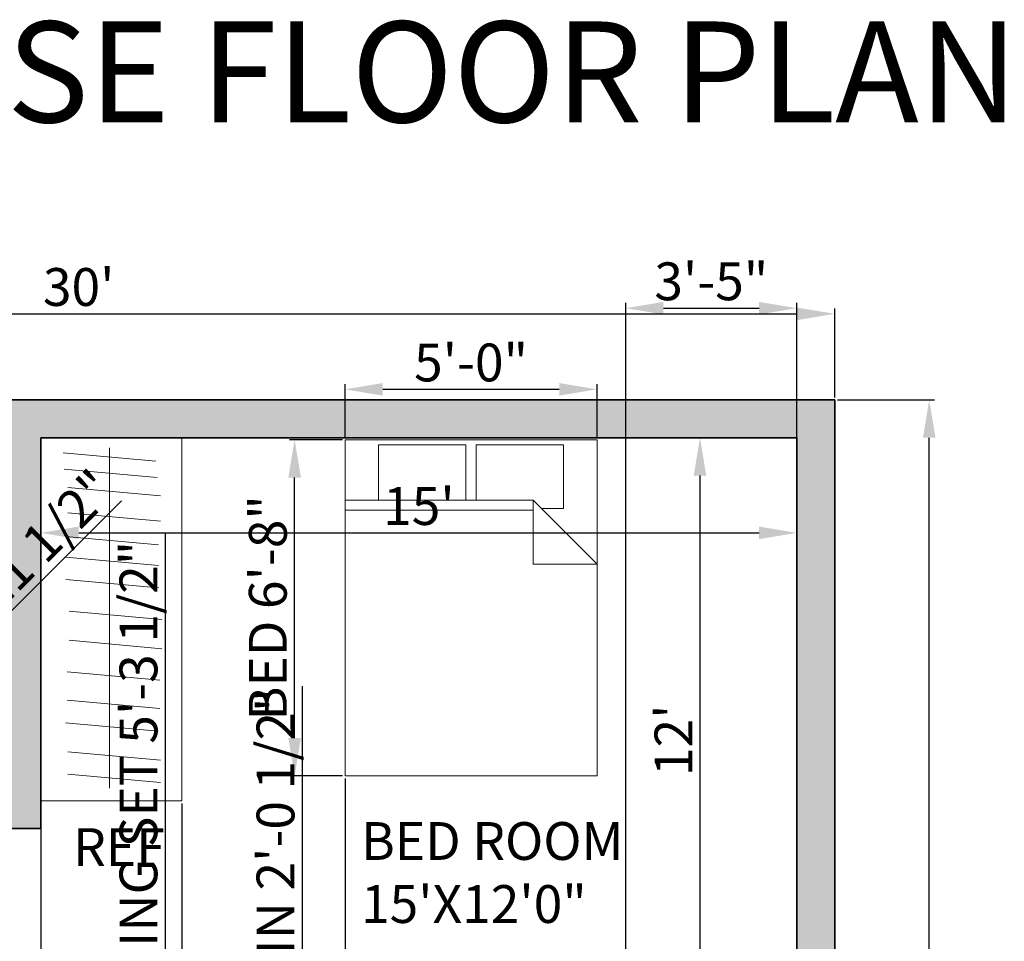
# Model space of a CAD drawing. Units: inches. Extents: x 39700 to 40173, y 40700 to 41139.
# Tile 4 of 4: x 39899 to 40134, y 40919 to 41139. Entities that reach past the tile are written whole.
import ezdxf

# ---------------------------------------------------------------- set-up
doc = ezdxf.new("R2010")
doc.units = ezdxf.units.IN
for name, color, linetype, lineweight in [('A-ANNO-DIMS', 2, 'Continuous', 18), ('A-ANNO-TEXT', 7, 'Continuous', 25), ('A-AREA-IDEN', 7, 'Continuous', 25), ('A-FLOR-CABN', 9, 'Continuous', 18), ('A-FURN', 8, 'Continuous', 18), ('A-WALL', 7, 'Continuous', 35)]:
    doc.layers.add(name, color=color, linetype=linetype, lineweight=lineweight)
doc.layers.add('A-WALL-PATT', color=251, linetype='Continuous', lineweight=13, true_color=0x636466)
doc.styles.get("Standard").update_dxf_attribs({"font": 'arial.ttf'})
doc.dimstyles.new('ISO-25', dxfattribs={"dimtxt": 9, "dimasz": 9, "dimexe": 1.25, "dimexo": 0.625, "dimtad": 1, "dimdec": 1, "dimrnd": 9, "dimlunit": 3, "dimtxsty": 'Standard', "dimcen": 2.5, "dimadec": 0, "dimazin": 0, "dimtfac": 1, "dimtdec": 1, "dimtmove": 0, "dimatfit": 3, "dimfxl": 1, "dimarcsym": 0})

# ---------------------------------------------------------------- blocks, each defined once
blk = doc.blocks.new('*D5')
at = {"layer": 'A-ANNO-DIMS', "color": 0, "lineweight": -2, "transparency": 16777216}
for p, q in [((39904.42, 41038.42), (39904.42, 41015.16)), ((40084.42, 41038.42), (40084.42, 41015.16)), ((39913.42, 41016.41), (40075.42, 41016.41))]:
    blk.add_line(p, q, dxfattribs=at)
at = {"layer": 'A-ANNO-DIMS', "color": 0, "transparency": 16777216}
for points in [[(39913.42, 41017.91), (39913.42, 41014.91), (39904.42, 41016.41)], [(40075.42, 41017.91), (40075.42, 41014.91), (40084.42, 41016.41)]]:
    blk.add_solid(points, dxfattribs=at)
at = {"layer": 'Defpoints', "color": 0, "transparency": 16777216}
for p in [(39904.42, 41039.04), (40084.42, 41039.04), (40084.42, 41016.41)]:
    blk.add_point(p, dxfattribs=at)
at = {"layer": 'A-ANNO-DIMS', "color": 0, "transparency": 16777216, "insert": (39994.42, 41021.63), "char_height": 9, "attachment_point": 5}
blk.add_mtext("15'", dxfattribs=at)
blk = doc.blocks.new('*D6')
at = {"layer": 'A-ANNO-DIMS', "color": 0, "lineweight": -2, "transparency": 16777216}
for p, q in [((40083.8, 41039.04), (40060.09, 41039.04)), ((40061.34, 41030.04), (40061.34, 40904.04)), ((40083.8, 40895.04), (40060.09, 40895.04))]:
    blk.add_line(p, q, dxfattribs=at)
at = {"layer": 'A-ANNO-DIMS', "color": 0, "transparency": 16777216}
for points in [[(40059.84, 41030.04), (40062.84, 41030.04), (40061.34, 41039.04)], [(40059.84, 40904.04), (40062.84, 40904.04), (40061.34, 40895.04)]]:
    blk.add_solid(points, dxfattribs=at)
at = {"layer": 'Defpoints', "color": 0, "transparency": 16777216}
for p in [(40084.42, 41039.04), (40061.34, 40895.04), (40084.42, 40895.04)]:
    blk.add_point(p, dxfattribs=at)
at = {"layer": 'A-ANNO-DIMS', "color": 0, "transparency": 16777216, "insert": (40056.19, 40967.04), "char_height": 9, "attachment_point": 5, "rotation": 90}
blk.add_mtext("12'", dxfattribs=at)
blk = doc.blocks.new('*D9')
at = {"layer": 'A-ANNO-DIMS', "color": 0, "lineweight": -2, "transparency": 16777216}
for p, q in [((39733.42, 41048.67), (39733.42, 41069.8)), ((40093.42, 41048.67), (40093.42, 41069.8)), ((39742.42, 41068.55), (40084.42, 41068.55))]:
    blk.add_line(p, q, dxfattribs=at)
at = {"layer": 'A-ANNO-DIMS', "color": 0, "transparency": 16777216}
for points in [[(39742.42, 41070.05), (39742.42, 41067.05), (39733.42, 41068.55)], [(40084.42, 41070.05), (40084.42, 41067.05), (40093.42, 41068.55)]]:
    blk.add_solid(points, dxfattribs=at)
at = {"layer": 'Defpoints', "color": 0, "transparency": 16777216}
for p in [(40093.42, 41068.55), (39733.42, 41048.04), (40093.42, 41048.04)]:
    blk.add_point(p, dxfattribs=at)
at = {"layer": 'A-ANNO-DIMS', "color": 0, "transparency": 16777216, "insert": (39913.42, 41073.77), "char_height": 9, "attachment_point": 5}
blk.add_mtext("30'", dxfattribs=at)
blk = doc.blocks.new('*D10')
at = {"layer": 'A-ANNO-DIMS', "color": 0, "lineweight": -2, "transparency": 16777216}
for p, q in [((40094.05, 41048.04), (40117.17, 41048.04)), ((40115.92, 40757.04), (40115.92, 41039.04)), ((40094.05, 40748.04), (40117.17, 40748.04))]:
    blk.add_line(p, q, dxfattribs=at)
at = {"layer": 'A-ANNO-DIMS', "color": 0, "transparency": 16777216}
for points in [[(40114.42, 41039.04), (40117.42, 41039.04), (40115.92, 41048.04)], [(40114.42, 40757.04), (40117.42, 40757.04), (40115.92, 40748.04)]]:
    blk.add_solid(points, dxfattribs=at)
at = {"layer": 'Defpoints', "color": 0, "transparency": 16777216}
for p in [(40093.42, 41048.04), (40115.92, 41048.04), (40093.42, 40748.04)]:
    blk.add_point(p, dxfattribs=at)
at = {"layer": 'A-ANNO-DIMS', "color": 0, "transparency": 16777216, "insert": (40110.7, 40898.04), "char_height": 9, "attachment_point": 5, "rotation": 90}
blk.add_mtext('25\'0"', dxfattribs=at)
blk = doc.blocks.new('Bed - Queen')
for p, q in [((0, -80.00003), (0, 0)), ((0, 0), (59.99999, 0)), ((59.99999, 0), (59.99999, -80.00003)), ((7.99999, -1.2), (28.79998, -1.2)), ((7.99999, -14.4), (7.99999, -1.2)), ((28.79998, -1.2), (28.79998, -14.4)), ((31.19999, -1.2), (51.99999, -1.2)), ((31.19999, -14.4), (31.19999, -1.2)), ((51.99999, -1.2), (51.99999, -16.4)), ((0, -14.4), (44.8, -14.4)), ((59.99999, -29.6), (44.8, -14.4)), ((44.8, -14.4), (44.8, -29.6)), ((51.99999, -16.4), (46.79936, -16.4)), ((44.8, -16.8), (0, -16.8)), ((44.8, -29.6), (59.99999, -29.6)), ((59.99999, -80.00003), (0, -80.00003))]:
    blk.add_line(p, q)
blk = doc.blocks.new('*D24')
at = {"layer": 'A-ANNO-DIMS', "color": 0, "lineweight": -2, "transparency": 16777216}
for p, q in [((39976.2, 41038.58), (39963.58, 41038.58)), ((39964.83, 40967.58), (39964.83, 41029.58)), ((39976.2, 40958.58), (39963.58, 40958.58))]:
    blk.add_line(p, q, dxfattribs=at)
at = {"layer": 'A-ANNO-DIMS', "color": 0, "transparency": 16777216}
for points in [[(39963.33, 41029.58), (39966.33, 41029.58), (39964.83, 41038.58)], [(39963.33, 40967.58), (39966.33, 40967.58), (39964.83, 40958.58)]]:
    blk.add_solid(points, dxfattribs=at)
at = {"layer": 'Defpoints', "color": 0, "transparency": 16777216}
for p in [(39964.83, 41038.58), (39976.83, 41038.58), (39976.83, 40958.58)]:
    blk.add_point(p, dxfattribs=at)
at = {"layer": 'A-ANNO-DIMS', "color": 0, "transparency": 16777216, "insert": (39959.61, 40998.58), "char_height": 9, "attachment_point": 5, "rotation": 90}
blk.add_mtext('BED 6\'-8"', dxfattribs=at)
blk = doc.blocks.new('*D25')
at = {"layer": 'A-ANNO-DIMS', "color": 0, "lineweight": -2, "transparency": 16777216}
for p, q in [((39976.83, 41039.21), (39976.83, 41051.83)), ((40036.83, 41039.21), (40036.83, 41051.83)), ((39985.83, 41050.58), (40027.83, 41050.58))]:
    blk.add_line(p, q, dxfattribs=at)
at = {"layer": 'A-ANNO-DIMS', "color": 0, "transparency": 16777216}
for points in [[(39985.83, 41052.08), (39985.83, 41049.08), (39976.83, 41050.58)], [(40027.83, 41052.08), (40027.83, 41049.08), (40036.83, 41050.58)]]:
    blk.add_solid(points, dxfattribs=at)
at = {"layer": 'Defpoints', "color": 0, "transparency": 16777216}
for p in [(40036.83, 41050.58), (39976.83, 41038.58), (40036.83, 41038.58)]:
    blk.add_point(p, dxfattribs=at)
at = {"layer": 'A-ANNO-DIMS', "color": 0, "transparency": 16777216, "insert": (40006.83, 41055.8), "char_height": 9, "attachment_point": 5}
blk.add_mtext('5\'-0"', dxfattribs=at)
blk = doc.blocks.new('*D30')
at = {"layer": 'A-ANNO-DIMS', "color": 0, "lineweight": -2, "transparency": 16777216}
for p, q in [((39934.09, 40886.16), (39934.09, 41016.31)), ((39925.16, 40886.16), (39935.34, 40886.16)), ((39934.09, 40831.46), (39934.09, 40877.16)), ((39925.16, 40822.46), (39935.34, 40822.46))]:
    blk.add_line(p, q, dxfattribs=at)
at = {"layer": 'A-ANNO-DIMS', "color": 0, "transparency": 16777216}
for points in [[(39932.59, 40877.16), (39935.59, 40877.16), (39934.09, 40886.16)], [(39932.59, 40831.46), (39935.59, 40831.46), (39934.09, 40822.46)]]:
    blk.add_solid(points, dxfattribs=at)
at = {"layer": 'Defpoints', "color": 0, "transparency": 16777216}
for p in [(39924.53, 40886.16), (39934.09, 40886.16), (39924.53, 40822.46)]:
    blk.add_point(p, dxfattribs=at)
at = {"layer": 'A-ANNO-DIMS', "color": 0, "transparency": 16777216, "insert": (39928.81, 40955.74), "char_height": 9, "attachment_point": 5, "rotation": 90}
blk.add_mtext('DINING SET 5\'-3 1/2"', dxfattribs=at)
blk = doc.blocks.new('*D38')
at = {"layer": 'A-ANNO-DIMS', "color": 0, "lineweight": -2, "transparency": 16777216}
for p, q in [((39966.72, 40883.91), (39966.72, 40979.88)), ((39969.78, 40883.91), (39965.47, 40883.91)), ((39966.72, 40868.36), (39966.72, 40874.91)), ((39969.78, 40859.36), (39965.47, 40859.36))]:
    blk.add_line(p, q, dxfattribs=at)
at = {"layer": 'A-ANNO-DIMS', "color": 0, "transparency": 16777216}
for points in [[(39965.22, 40874.91), (39968.22, 40874.91), (39966.72, 40883.91)], [(39965.22, 40868.36), (39968.22, 40868.36), (39966.72, 40859.36)]]:
    blk.add_solid(points, dxfattribs=at)
at = {"layer": 'Defpoints', "color": 0, "transparency": 16777216}
for p in [(39966.72, 40883.91), (39970.4, 40883.91), (39970.4, 40859.36)]:
    blk.add_point(p, dxfattribs=at)
at = {"layer": 'A-ANNO-DIMS', "color": 0, "transparency": 16777216, "insert": (39961.44, 40936.4), "char_height": 9, "attachment_point": 5, "rotation": 90}
blk.add_mtext('BASIN 2\'-0 1/2"', dxfattribs=at)
blk = doc.blocks.new('*D47')
at = {"layer": 'A-ANNO-DIMS', "color": 0, "lineweight": -2, "transparency": 16777216}
for p, q in [((40043.65, 40858.83), (40043.65, 41071.14)), ((40052.65, 41069.89), (40075.42, 41069.89)), ((40084.42, 40858.83), (40084.42, 41071.14))]:
    blk.add_line(p, q, dxfattribs=at)
at = {"layer": 'A-ANNO-DIMS', "color": 0, "transparency": 16777216}
for points in [[(40052.65, 41071.39), (40052.65, 41068.39), (40043.65, 41069.89)], [(40075.42, 41071.39), (40075.42, 41068.39), (40084.42, 41069.89)]]:
    blk.add_solid(points, dxfattribs=at)
at = {"layer": 'Defpoints', "color": 0, "transparency": 16777216}
for p in [(40084.42, 41069.89), (40043.65, 40858.21), (40084.42, 40858.21)]:
    blk.add_point(p, dxfattribs=at)
at = {"layer": 'A-ANNO-DIMS', "color": 0, "transparency": 16777216, "insert": (40064.03, 41075.12), "char_height": 9, "attachment_point": 5}
blk.add_mtext('3\'-5"', dxfattribs=at)
blk = doc.blocks.new('*D50')
at = {"layer": 'A-ANNO-DIMS', "color": 0, "lineweight": -2, "transparency": 16777216}
for p, q in [((39904.42, 40952.02), (39904.42, 40724.94)), ((39937.94, 40952.02), (39937.94, 40724.94)), ((39913.42, 40726.19), (39928.94, 40726.19)), ((39937.94, 40726.19), (39993.24, 40726.19))]:
    blk.add_line(p, q, dxfattribs=at)
at = {"layer": 'A-ANNO-DIMS', "color": 0, "transparency": 16777216}
for points in [[(39913.42, 40727.69), (39913.42, 40724.69), (39904.42, 40726.19)], [(39928.94, 40727.69), (39928.94, 40724.69), (39937.94, 40726.19)]]:
    blk.add_solid(points, dxfattribs=at)
at = {"layer": 'Defpoints', "color": 0, "transparency": 16777216}
for p in [(39904.42, 40952.64), (39937.94, 40952.64), (39937.94, 40726.19)]:
    blk.add_point(p, dxfattribs=at)
at = {"layer": 'A-ANNO-DIMS', "color": 0, "transparency": 16777216, "insert": (39970.09, 40731.47), "char_height": 9, "attachment_point": 5}
blk.add_mtext('2\'-9 1/2"', dxfattribs=at)
blk = doc.blocks.new('*D51')
at = {"layer": 'A-ANNO-DIMS', "color": 0, "lineweight": -2, "transparency": 16777216}
for p, q in [((39976.83, 40957.96), (39976.83, 40724.94)), ((39937.94, 40952.02), (39937.94, 40724.94)), ((39946.94, 40726.19), (39967.83, 40726.19))]:
    blk.add_line(p, q, dxfattribs=at)
at = {"layer": 'A-ANNO-DIMS', "color": 0, "transparency": 16777216}
for points in [[(39946.94, 40727.69), (39946.94, 40724.69), (39937.94, 40726.19)], [(39967.83, 40727.69), (39967.83, 40724.69), (39976.83, 40726.19)]]:
    blk.add_solid(points, dxfattribs=at)
at = {"layer": 'Defpoints', "color": 0, "transparency": 16777216}
for p in [(39976.83, 40958.58), (39937.94, 40952.64), (39976.83, 40726.19)]:
    blk.add_point(p, dxfattribs=at)
at = {"layer": 'A-ANNO-DIMS', "color": 0, "transparency": 16777216, "insert": (39957.39, 40731.42), "char_height": 9, "attachment_point": 5}
blk.add_mtext('3\'-3"', dxfattribs=at)
blk = doc.blocks.new('*D54')
at = {"layer": 'A-ANNO-DIMS', "color": 0, "lineweight": -2, "transparency": 16777216}
for p, q in [((39923.61, 41024.06), (39873.58, 40974.03)), ((39850.6, 40951.04), (39867.22, 40967.66))]:
    blk.add_line(p, q, dxfattribs=at)
at = {"layer": 'A-ANNO-DIMS', "color": 0, "transparency": 16777216}
blk.add_solid([(39872.52, 40975.09), (39874.64, 40972.97), (39867.22, 40967.66)], dxfattribs=at)
at = {"layer": 'Defpoints', "color": 0, "transparency": 16777216}
for p in [(39867.22, 40967.66), (39850.6, 40951.04)]:
    blk.add_point(p, dxfattribs=at)
at = {"layer": 'A-ANNO-DIMS', "color": 0, "transparency": 16777216, "insert": (39898.05, 41005.96), "char_height": 9, "attachment_point": 5, "rotation": 44.999}
blk.add_mtext('R1\'-11 1/2"', dxfattribs=at)

msp = doc.modelspace()

# ---------------------------------------------------------------- hatches: boundary and pattern name
at = {"layer": 'A-WALL-PATT'}
h = msp.add_hatch(color=256, dxfattribs=at)
h.dxf.hatch_style = 1
h.paths.add_polyline_path([(39742.42, 41039.04), (39838.42, 41039.04), (39838.42, 40943.28, -0.039113), (39842.92, 40942.53), (39847.42, 40942.53), (39847.42, 40946.04), (39850.1, 40946.04), (39850.1, 40955.04), (39847.42, 40955.04), (39847.42, 41039.04), (39895.42, 41039.04), (39895.42, 40955.04), (39874.1, 40955.04), (39874.1, 40951.54, -0.010637), (39874.1, 40950.54), (39874.1, 40946.04), (39895.42, 40946.04), (39904.42, 40946.04), (39904.42, 41039.04), (40084.42, 41039.04), (40084.42, 40895.04), (39960.51, 40895.04), (39960.51, 40886.04), (40084.42, 40886.04), (40084.42, 40817.04), (40093.42, 40817.04), (40093.42, 41048.04), (39733.42, 41048.04), (39733.42, 40889.95), (39742.42, 40889.95)])
h.paths.add_polyline_path([(39742.42, 40841.95), (39733.42, 40841.95), (39733.42, 40817.06), (39737.92, 40817.06, -0.015901), (39740.88, 40817.06), (39742.42, 40817.06)], flags=17)
h.paths.add_polyline_path([(40093.42, 40757.04), (39796.66, 40757.04), (39796.66, 40748.04), (40093.42, 40748.04)])
h.paths.add_polyline_path([(39753.27, 40757.04), (39742.42, 40757.04), (39742.42, 40769.06), (39733.42, 40769.06), (39733.42, 40748.04), (39753.27, 40748.04)])
h.paths.add_polyline_path([(40084.42, 40826.04), (39960.51, 40826.04), (39960.51, 40817.04), (40084.42, 40817.04)], flags=17)
h.paths.add_polyline_path([(39969.51, 40859.86), (39960.51, 40859.86), (39960.51, 40852.78), (39969.51, 40852.78)], flags=17)
h.paths.add_polyline_path([(39969.51, 40886.04), (39960.51, 40886.04), (39960.51, 40881.75), (39969.51, 40881.75)], flags=17)
h.paths.add_polyline_path([(39852.31, 40989.98), (39900.82, 40989.98), (39900.82, 41008.52), (39852.31, 41008.52)], flags=25)

# ---------------------------------------------------------------- linework, layer by layer
at = {"layer": 'A-FLOR-CABN'}
for p, q in [((39937.94, 41039.04), (39937.94, 40952.64)), ((39909.74, 41035.44), (39931.81, 41033.45)), ((39920.78, 41036.66), (39920.78, 40955.64)), ((39910, 41031.55), (39932.07, 41029.56)), ((39910.86, 41027.22), (39932.93, 41025.23)), ((39910.86, 41021.15), (39932.93, 41019.17)), ((39910.36, 41015.55), (39932.43, 41013.56)), ((39910.36, 41010.6), (39932.43, 41008.62)), ((39910.36, 41005.33), (39932.43, 41003.34)), ((39911.12, 40997.75), (39933.19, 40995.76)), ((39911.12, 40990.83), (39933.19, 40988.84)), ((39910.7, 40983.36), (39932.77, 40981.37)), ((39910.7, 40976.58), (39932.77, 40974.59)), ((39910.29, 40971.18), (39932.36, 40969.2)), ((39910.84, 40964.27), (39932.91, 40962.28)), ((39910.84, 40959.01), (39932.91, 40957.02)), ((39937.94, 40952.64), (39904.42, 40952.64))]:
    msp.add_line(p, q, dxfattribs=at)
at = {"layer": 'A-WALL'}
for p, q in [((40093.42, 41048.04), (39733.42, 41048.04)), ((40093.42, 40748.04), (40093.42, 41048.04)), ((40084.42, 41039.04), (39904.42, 41039.04)), ((39904.42, 41039.04), (39904.42, 40946.04)), ((40084.42, 40895.04), (40084.42, 41039.04)), ((39904.42, 40946.04), (39895.42, 40946.04))]:
    msp.add_line(p, q, dxfattribs=at)

# ---------------------------------------------------------------- block references
at = {"layer": 'A-FURN'}
msp.add_blockref('Bed - Queen', (39976.83, 41038.58), dxfattribs=at)

# ---------------------------------------------------------------- texts
at = {"layer": 'A-ANNO-TEXT', "attachment_point": 1}
for s, width, insert, char_height in [('1BHK HOUSE FLOOR PLAN', 457.4103, (39732.57, 41138.14), 24), ('REF', 23.7932, (39912.09, 40946.11), 9)]:
    msp.add_mtext_dynamic_manual_height_columns(s, width=width, gutter_width=12.5, heights=[0], dxfattribs=dict(at, insert=insert, char_height=char_height))
at = {"layer": 'A-AREA-IDEN', "insert": (39980.63, 40947.56), "char_height": 9, "attachment_point": 1}
msp.add_mtext_dynamic_manual_height_columns('BED ROOM\\P15\'X12\'0"', width=81.6943, gutter_width=12.5, heights=[0], dxfattribs=at)

# ---------------------------------------------------------------- dimensions: what is measured, and where the dimension line sits
at = {"layer": 'A-ANNO-DIMS'}
for base, p1, p2, override, picture, middle in [((40093.42, 41068.55), (39733.42, 41048.04), (40093.42, 41048.04), {"dimclrd": 0, "dimclre": 0, "dimclrt": 0}, '*D9', (39913.42, 41073.77)), ((40084.42, 41069.89), (40043.65, 40858.21), (40084.42, 40858.21), {"dimdec": 1, "dimlfac": 1, "dimrnd": 0, "dimzin": 1, "dimdsep": 46, "dimlunit": 4, "dimfrac": 2}, '*D47', (40064.03, 41075.12)), ((40036.83, 41050.58), (39976.83, 41038.58), (40036.83, 41038.58), {"dimdec": 1, "dimlfac": 1, "dimrnd": 0, "dimzin": 1, "dimdsep": 46, "dimlunit": 4, "dimfrac": 2}, '*D25', (40006.83, 41055.8)), ((40084.42, 41016.41), (39904.42, 41039.04), (40084.42, 41039.04), {"dimclrd": 0, "dimclre": 0, "dimclrt": 0}, '*D5', (39994.42, 41021.63)), ((39976.83, 40726.19), (39937.94, 40952.64), (39976.83, 40958.58), {"dimdec": 1, "dimlfac": 1, "dimrnd": 0, "dimzin": 1, "dimdsep": 46, "dimlunit": 4, "dimfrac": 2}, '*D51', (39957.39, 40731.42)), ((39937.94, 40726.19), (39904.42, 40952.64), (39937.94, 40952.64), {"dimdec": 1, "dimlfac": 1, "dimrnd": 0, "dimzin": 1, "dimdsep": 46, "dimlunit": 4, "dimfrac": 2}, '*D50', (39970.09, 40731.47))]:
    dim = msp.add_linear_dim(base=base, p1=p1, p2=p2, dimstyle='ISO-25', override=override, dxfattribs=at)
    dim.commit()
    dim.dimension.update_dxf_attribs({"geometry": picture, "text_midpoint": middle})
for base, p1, p2, text, override, picture, middle in [((40115.92, 41048.04), (40093.42, 40748.04), (40093.42, 41048.04), '25\'0"', {"dimclrd": 0, "dimclre": 0, "dimclrt": 0}, '*D10', (40110.7, 40898.04)), ((39964.83, 41038.58), (39976.83, 40958.58), (39976.83, 41038.58), 'BED <>', {"dimdec": 1, "dimlfac": 1, "dimrnd": 0, "dimzin": 1, "dimdsep": 46, "dimlunit": 4, "dimfrac": 2}, '*D24', (39959.61, 40998.58)), ((39934.09, 40886.16), (39924.53, 40822.46), (39924.53, 40886.16), 'DINING SET <>', {"dimdec": 1, "dimlfac": 1, "dimrnd": 0, "dimzin": 1, "dimdsep": 46, "dimlunit": 4, "dimfrac": 2}, '*D30', (39928.81, 40955.74)), ((39966.7205, 40883.9107), (39970.4032, 40859.3598), (39970.4032, 40883.9107), 'BASIN <>', {"dimdec": 1, "dimlfac": 1, "dimrnd": 0, "dimzin": 1, "dimdsep": 46, "dimlunit": 4, "dimfrac": 2}, '*D38', (39961.442, 40936.3962))]:
    dim = msp.add_linear_dim(base=base, p1=p1, p2=p2, angle=90, text=text, dimstyle='ISO-25', override=override, dxfattribs=at)
    dim.commit()
    dim.dimension.update_dxf_attribs({"geometry": picture, "text_midpoint": middle})
dim = msp.add_linear_dim(base=(40061.34, 40895.04), p1=(40084.42, 41039.04), p2=(40084.42, 40895.04), angle=90, dimstyle='ISO-25', override={"dimclrd": 0, "dimclre": 0, "dimclrt": 0}, dxfattribs=at)
dim.commit()
dim.dimension.update_dxf_attribs({"geometry": '*D6', "text_midpoint": (40056.19, 40967.04)})
dim = msp.add_radius_dim(center=(39850.6, 40951.04), mpoint=(39867.22, 40967.66), dimstyle='ISO-25', override={"dimdec": 1, "dimlfac": 1, "dimrnd": 0, "dimzin": 1, "dimdsep": 46, "dimlunit": 4, "dimfrac": 2}, dxfattribs=at)
dim.commit()
dim.dimension.update_dxf_attribs({"geometry": '*D54', "text_midpoint": (39898.05, 41005.96)})

doc.saveas('drawing.dxf')
